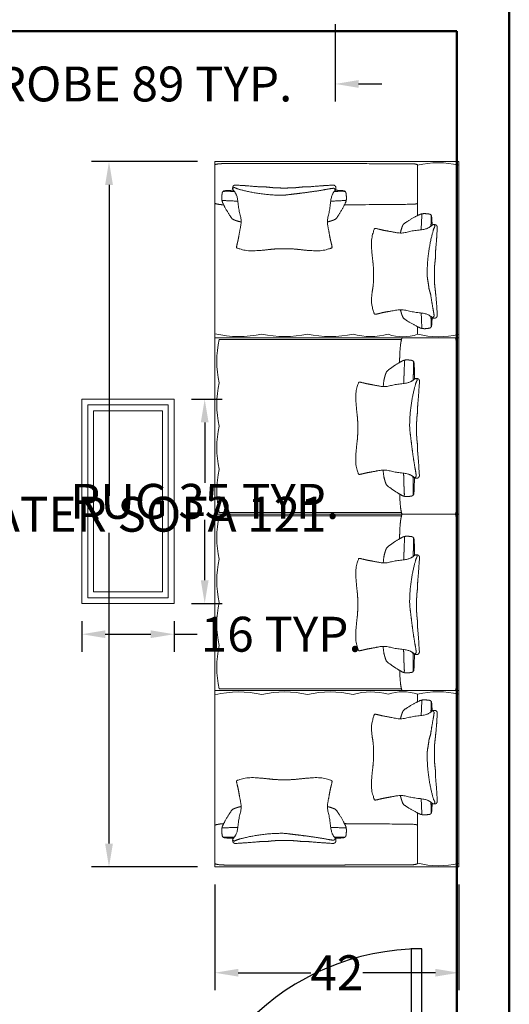
# Model space of a CAD drawing. Units: inches. Extents: x -466983 to 1020, y 324 to 318697.
# Tile 40 of 97: x 908 to 992, y 658 to 827. Entities that reach past the tile are written whole.
import ezdxf

# ---------------------------------------------------------------- set-up
doc = ezdxf.new("R2010")
doc.units = ezdxf.units.IN
doc.header["$MEASUREMENT"] = 0
for name, color, linetype, lineweight in [('A-ANNO-DIMS', 2, 'Continuous', 18), ('A-DOOR', 3, 'Continuous', 25), ('A-FURN', 8, 'Continuous', 18), ('A-WALL', 7, 'Continuous', 50)]:
    doc.layers.add(name, color=color, linetype=linetype, lineweight=lineweight)
doc.styles.get("Standard").update_dxf_attribs({"font": 'arial.ttf'})
doc.dimstyles.get("Standard").update_dxf_attribs({"dimtxt": 6, "dimasz": 4, "dimexe": 3, "dimexo": 3, "dimgap": 0.09, "dimtad": 0, "dimtih": 1, "dimtoh": 1, "dimdec": 1, "dimzin": 0, "dimdsep": 46, "dimlunit": 3, "dimtxsty": 'Standard', "dimcen": 0.09, "dimadec": 0, "dimazin": 0, "dimtfac": 1, "dimtdec": 1, "dimtofl": 0, "dimtmove": 0, "dimatfit": 3, "dimfxl": 1, "dimtolj": 1, "dimtzin": 0, "dimarcsym": 0})

# ---------------------------------------------------------------- blocks, each defined once
blk = doc.blocks.new('4 Seater Sofa Drawing')
for p, q in [((2474.13, 1022.64), (2521.12, 1022.64)), ((2474.13, 957.71), (2474.13, 1022.64)), ((2474.13, 1022.64), (2521.12, 1022.64)), ((2474.13, 957.71), (2474.13, 1022.64)), ((2568.11, 1022.64), (2521.12, 1022.64)), ((2521.12, 1022.64), (2521.12, 957.71)), ((2521.12, 1022.64), (2521.12, 957.71)), ((2521.12, 1022.64), (2521.12, 957.71)), ((2568.11, 957.71), (2568.11, 1022.64)), ((2615.09, 1022.64), (2568.11, 1022.64)), ((2568.11, 1022.64), (2568.11, 957.71)), ((2615.09, 957.71), (2615.09, 1022.64)), ((2662.08, 1022.64), (2615.09, 1022.64)), ((2615.09, 1022.64), (2615.09, 957.71)), ((2662.08, 957.71), (2662.08, 1022.64)), ((2485.15, 1011.7), (2488.51, 1011.7)), ((2518.14, 1011.7), (2520.13, 1011.7)), ((2618.07, 1011.7), (2616.08, 1011.7)), ((2651.06, 1011.7), (2647.71, 1011.7)), ((2521.57, 1007.39), (2521.57, 958.85)), ((2567.65, 1007.4), (2567.65, 986.81)), ((2568.56, 1007.39), (2568.56, 958.85)), ((2614.64, 1007.4), (2614.64, 986.81)), ((2567.65, 958.85), (2567.65, 986.81)), ((2614.64, 958.85), (2614.64, 986.81)), ((2521.12, 957.71), (2474.13, 957.71)), ((2521.12, 957.71), (2474.13, 957.71)), ((2521.12, 957.71), (2568.11, 957.71)), ((2568.11, 957.71), (2615.09, 957.71)), ((2615.09, 957.71), (2662.08, 957.71))]:
    blk.add_line(p, q)
at = {"extrusion": (0, 0, -1)}
for p, q in [((2568.11, 1022.64), (2521.12, 1022.64)), ((2521.12, 1022.64), (2521.12, 957.71)), ((2568.11, 957.71), (2568.11, 1022.64)), ((2615.09, 1022.64), (2568.11, 1022.64)), ((2568.11, 1022.64), (2568.11, 957.71)), ((2615.09, 957.71), (2615.09, 1022.64)), ((2662.08, 1022.64), (2615.09, 1022.64)), ((2615.09, 1022.64), (2615.09, 957.71)), ((2662.08, 957.71), (2662.08, 1022.64)), ((2521.12, 957.71), (2568.11, 957.71)), ((2568.11, 957.71), (2615.09, 957.71)), ((2615.09, 957.71), (2662.08, 957.71))]:
    blk.add_line(p, q, dxfattribs=at)
for centre, radius, start, end in [((2497.81, 1017.25), 23.36, 166.6748, 193.7611), ((2497.44, 1017.25), 23.36, 346.2389, 13.3252), ((2638.77, 1017.25), 23.36, 166.6748, 193.7611), ((2638.4, 1017.25), 23.36, 346.2389, 13.3252), ((2508.99, 1007.76), 11.82, 340.5487, 19.4513), ((2627.22, 1007.76), 11.82, 160.5487, 199.4513), ((2503.6, 999.25), 17.15, 343.8796, 15.4668), ((2632.61, 999.25), 17.15, 164.5332, 196.1204), ((2493.1, 988.42), 27.66, 347.3212, 12.6788), ((2643.12, 988.42), 27.66, 167.3212, 192.6788), ((2493.1, 976.28), 27.66, 347.3212, 12.6788), ((2643.12, 976.28), 27.66, 167.3212, 192.6788), ((2493.1, 964.14), 27.66, 346.5695, 12.6788), ((2643.12, 964.14), 27.66, 167.3212, 193.4305), ((2527.33, 984.45), 26.24, 257.3212, 282.6788), ((2538.86, 984.48), 26.27, 257.3272, 282.6647), ((2550.37, 984.48), 26.27, 257.3353, 282.6728), ((2561.9, 984.45), 26.24, 257.3212, 282.6788), ((2574.32, 984.45), 26.24, 257.3212, 282.6788), ((2585.84, 984.48), 26.27, 257.3272, 282.6647), ((2597.36, 984.48), 26.27, 257.3353, 282.6728), ((2608.88, 984.45), 26.24, 257.3212, 282.6788)]:
    blk.add_arc(centre, radius, start, end)
for points in [[(2522.19, 1022), (2521.12, 1021.86), (2521.12, 1021.69)], [(2521.12, 1021.69), (2521.12, 1012.51), (2521.12, 1007.6)], [(2530.42, 1022.1), (2524.11, 1022.1), (2523.25, 1022.08), (2522.69, 1022.05), (2522.19, 1022)], [(2539.72, 1022.1), (2535.07, 1022.1), (2530.42, 1022.1)], [(2558.8, 1022.1), (2549.26, 1022.1), (2539.72, 1022.1)], [(2567.04, 1022), (2566.54, 1022.05), (2565.98, 1022.08), (2565.12, 1022.1), (2558.8, 1022.1)], [(2568.11, 1021.69), (2568.11, 1021.86), (2567.04, 1022)], [(2569.17, 1022), (2568.11, 1021.86), (2568.11, 1021.69)], [(2568.11, 1007.6), (2568.11, 1012.51), (2568.11, 1021.69)], [(2568.11, 1021.69), (2568.11, 1012.51), (2568.11, 1007.6)], [(2577.41, 1022.1), (2571.1, 1022.1), (2570.23, 1022.08), (2569.67, 1022.05), (2569.17, 1022)], [(2586.7, 1022.1), (2582.06, 1022.1), (2577.41, 1022.1)], [(2605.79, 1022.1), (2596.25, 1022.1), (2586.7, 1022.1)], [(2614.03, 1022), (2613.53, 1022.05), (2612.97, 1022.08), (2612.1, 1022.1), (2605.79, 1022.1)], [(2615.09, 1021.69), (2615.09, 1021.86), (2614.03, 1022)], [(2615.09, 1007.6), (2615.09, 1012.51), (2615.09, 1021.69)], [(2501.5, 999.85), (2500.87, 999.78), (2498.56, 999.52), (2494.94, 999.32), (2492.12, 1000.1), (2491.9, 1000.31), (2492.12, 1001.33), (2492.44, 1002.59), (2492.75, 1004.42), (2493.33, 1007.39), (2492.57, 1010.18), (2492.19, 1013.75), (2491.52, 1015.06), (2490.91, 1015.73), (2490.9, 1016.23), (2491.01, 1016.65), (2491.47, 1016.97), (2491.84, 1016.93)], [(2491.37, 1016.31), (2491.29, 1016.29), (2490.91, 1016.08)], [(2491.84, 1016.93), (2493.92, 1016.78), (2494.29, 1016.78), (2497.41, 1016.52), (2498.38, 1016.42), (2499.92, 1016.45), (2500.85, 1016.32)], [(2500.85, 1016.32), (2501.67, 1016.22), (2502.67, 1016.17)], [(2505.99, 1016.17), (2506.99, 1016.22), (2507.81, 1016.32)], [(2514.92, 1016.93), (2515.29, 1016.97), (2515.75, 1016.65), (2515.86, 1016.23), (2515.85, 1015.73), (2515.24, 1015.06), (2514.57, 1013.75), (2514.2, 1010.18), (2513.43, 1007.39), (2514.01, 1004.42), (2514.32, 1002.59), (2514.64, 1001.33), (2514.87, 1000.31), (2514.64, 1000.1), (2511.82, 999.32), (2509.24, 999.52), (2507.79, 999.78), (2507.16, 999.85)], [(2507.81, 1016.32), (2508.73, 1016.45), (2509.42, 1016.42), (2509.36, 1016.52), (2512.47, 1016.78), (2512.84, 1016.78), (2514.92, 1016.93)], [(2515.74, 1015.66), (2515.41, 1016.03), (2515.29, 1016.08)], [(2621.29, 1016.93), (2620.92, 1016.97), (2620.46, 1016.65), (2620.36, 1016.23), (2620.37, 1015.73), (2620.97, 1015.06), (2621.64, 1013.75), (2622.02, 1010.18), (2622.78, 1007.39), (2622.2, 1004.42), (2621.89, 1002.59), (2621.58, 1001.33), (2621.35, 1000.31), (2621.57, 1000.1), (2624.39, 999.32), (2626.97, 999.52), (2628.43, 999.78), (2629.06, 999.85)], [(2620.47, 1015.66), (2620.81, 1016.03), (2620.93, 1016.08)], [(2628.41, 1016.32), (2627.48, 1016.45), (2626.79, 1016.42), (2626.86, 1016.52), (2623.74, 1016.78), (2623.37, 1016.78), (2621.29, 1016.93)], [(2630.23, 1016.17), (2629.23, 1016.22), (2628.41, 1016.32)], [(2635.37, 1016.32), (2634.55, 1016.22), (2633.55, 1016.17)], [(2634.72, 999.85), (2635.35, 999.78), (2637.65, 999.52), (2641.28, 999.32), (2644.09, 1000.1), (2644.32, 1000.31), (2644.09, 1001.33), (2643.78, 1002.59), (2643.47, 1004.42), (2642.89, 1007.39), (2643.65, 1010.18), (2644.03, 1013.75), (2644.69, 1015.06), (2645.3, 1015.73), (2645.31, 1016.23), (2645.21, 1016.65), (2644.74, 1016.97), (2644.38, 1016.93)], [(2644.38, 1016.93), (2642.3, 1016.78), (2641.93, 1016.78), (2638.81, 1016.52), (2637.83, 1016.42), (2636.29, 1016.45), (2635.37, 1016.32)], [(2644.85, 1016.31), (2644.93, 1016.29), (2645.31, 1016.08)], [(2505.36, 1014.32), (2505.01, 1014.28), (2504.66, 1014.25)], [(2507.98, 1014.72), (2506.44, 1014.53), (2505.36, 1014.32)], [(2509.58, 1015.18), (2508.66, 1014.9), (2507.98, 1014.72)], [(2626.63, 1015.18), (2627.56, 1014.9), (2628.24, 1014.72)], [(2628.24, 1014.72), (2629.77, 1014.53), (2630.86, 1014.32)], [(2630.86, 1014.32), (2631.21, 1014.28), (2631.56, 1014.25)], [(2474.62, 984.72), (2474.62, 991.35), (2474.64, 992.25), (2474.67, 992.84), (2474.72, 1010.58)], [(2474.72, 1010.58), (2474.87, 1011.7), (2475.04, 1011.7)], [(2475.04, 1011.7), (2480.12, 1011.7), (2485.19, 1011.7)], [(2485.19, 1011.7), (2485.33, 1011.7), (2485.46, 1010.93)], [(2485.46, 1010.93), (2485.55, 1010.63), (2485.64, 992.78)], [(2488.12, 1012.61), (2488.12, 1012.58), (2488.13, 1012.54)], [(2518.53, 1012.61), (2518.53, 1012.58), (2518.52, 1012.54)], [(2542.13, 995.65), (2541.53, 995.58), (2539.29, 995.34), (2535.79, 995.15), (2533.06, 995.91), (2532.85, 996.11), (2533.07, 997.1), (2533.37, 998.32), (2533.68, 1000.08), (2534.24, 1002.96), (2533.51, 1005.66), (2533.15, 1009.12), (2532.51, 1010.38), (2531.92, 1011.04), (2531.91, 1011.51), (2532.01, 1011.92), (2532.46, 1012.23), (2532.81, 1012.19)], [(2532.36, 1011.59), (2532.28, 1011.57), (2531.91, 1011.37)], [(2532.81, 1012.19), (2534.83, 1012.04), (2535.19, 1012.04), (2538.2, 1011.79), (2539.14, 1011.69), (2540.64, 1011.71), (2541.53, 1011.58)], [(2541.53, 1011.58), (2542.32, 1011.49), (2543.29, 1011.44)], [(2547.14, 1011.43), (2548.11, 1011.48), (2548.9, 1011.57)], [(2557.62, 1012.16), (2557.98, 1012.19), (2558.43, 1011.88), (2558.53, 1011.47), (2558.51, 1010.99), (2557.92, 1010.34), (2557.28, 1009.08), (2556.91, 1005.62), (2556.17, 1002.92), (2556.72, 1000.05), (2557.02, 998.28), (2557.32, 997.06), (2557.54, 996.07), (2557.32, 995.87), (2554.6, 995.12), (2551.09, 995.32), (2548.86, 995.57), (2548.25, 995.64)], [(2548.9, 1011.57), (2549.8, 1011.7), (2551.29, 1011.67), (2552.23, 1011.77), (2555.25, 1012.01), (2555.61, 1012.01), (2557.62, 1012.16)], [(2558.41, 1010.92), (2558.09, 1011.29), (2557.97, 1011.33)], [(2589.12, 995.65), (2588.51, 995.58), (2586.28, 995.34), (2582.77, 995.15), (2580.05, 995.91), (2579.83, 996.11), (2580.06, 997.1), (2580.36, 998.32), (2580.66, 1000.08), (2581.23, 1002.96), (2580.5, 1005.66), (2580.14, 1009.12), (2579.49, 1010.38), (2578.9, 1011.04), (2578.9, 1011.51), (2579, 1011.92), (2579.45, 1012.23), (2579.8, 1012.19)], [(2579.34, 1011.59), (2579.27, 1011.57), (2578.9, 1011.37)], [(2579.8, 1012.19), (2581.81, 1012.04), (2582.17, 1012.04), (2585.19, 1011.79), (2586.13, 1011.69), (2587.63, 1011.71), (2588.52, 1011.58)], [(2588.52, 1011.58), (2589.31, 1011.49), (2590.28, 1011.44)], [(2594.13, 1011.43), (2595.1, 1011.48), (2595.89, 1011.57)], [(2604.61, 1012.16), (2604.96, 1012.19), (2605.41, 1011.88), (2605.51, 1011.47), (2605.5, 1010.99), (2604.91, 1010.34), (2604.26, 1009.08), (2603.89, 1005.62), (2603.15, 1002.92), (2603.71, 1000.05), (2604.01, 998.28), (2604.31, 997.06), (2604.53, 996.07), (2604.31, 995.87), (2601.58, 995.12), (2598.08, 995.32), (2595.85, 995.57), (2595.24, 995.64)], [(2595.89, 1011.57), (2596.78, 1011.7), (2598.28, 1011.67), (2599.22, 1011.77), (2602.24, 1012.01), (2602.6, 1012.01), (2604.61, 1012.16)], [(2605.4, 1010.92), (2605.08, 1011.29), (2604.96, 1011.33)], [(2617.68, 1012.61), (2617.68, 1012.58), (2617.69, 1012.54)], [(2648.1, 1012.61), (2648.1, 1012.58), (2648.09, 1012.54)], [(2650.76, 1010.93), (2650.66, 1010.63), (2650.58, 992.78)], [(2651.03, 1011.7), (2650.88, 1011.7), (2650.76, 1010.93)], [(2661.17, 1011.7), (2656.1, 1011.7), (2651.03, 1011.7)], [(2661.49, 1010.58), (2661.34, 1011.7), (2661.17, 1011.7)], [(2661.6, 984.72), (2661.59, 991.35), (2661.58, 992.25), (2661.55, 992.84), (2661.49, 1010.58)], [(2521.12, 1007.6), (2521.12, 1007.47), (2521.84, 1007.34)], [(2527.1, 1008.02), (2527.1, 1007.99), (2527.11, 1007.95)], [(2563.27, 1007.96), (2563.27, 1007.94), (2563.26, 1007.89)], [(2567.38, 1007.34), (2568.11, 1007.47), (2568.11, 1007.6)], [(2568.11, 1007.6), (2568.11, 1007.47), (2568.83, 1007.34)], [(2574.09, 1008.02), (2574.09, 1007.99), (2574.1, 1007.95)], [(2610.26, 1007.96), (2610.26, 1007.94), (2610.25, 1007.89)], [(2614.37, 1007.34), (2615.09, 1007.47), (2615.09, 1007.6)], [(2484.71, 992.62), (2484.74, 992.62), (2484.78, 992.61)], [(2485.64, 992.78), (2485.67, 992.51), (2485.71, 992.19)], [(2650.58, 992.78), (2650.54, 992.51), (2650.51, 992.19)], [(2651.5, 992.62), (2651.48, 992.62), (2651.43, 992.61)], [(2480.39, 989.01), (2480.35, 989.38), (2480.67, 989.84), (2481.09, 989.95), (2481.59, 989.94), (2482.26, 989.33), (2483.57, 988.66), (2487.14, 988.29), (2489.93, 987.52), (2492.9, 988.1), (2494.73, 988.41), (2495.99, 988.73), (2497.01, 988.96), (2497.22, 988.73), (2498, 985.91), (2497.8, 982.29), (2497.54, 979.98), (2497.47, 979.35)], [(2481.66, 989.83), (2481.29, 989.5), (2481.24, 989.38)], [(2655.83, 989.01), (2655.87, 989.38), (2655.54, 989.84), (2655.12, 989.95), (2654.63, 989.94), (2653.95, 989.33), (2652.65, 988.66), (2649.07, 988.29), (2646.28, 987.52), (2643.31, 988.1), (2641.49, 988.41), (2640.23, 988.73), (2639.2, 988.96), (2639, 988.73), (2638.21, 985.91), (2638.41, 982.29), (2638.67, 979.98), (2638.74, 979.35)], [(2654.55, 989.83), (2654.93, 989.5), (2654.97, 989.38)], [(2481, 980), (2480.87, 980.93), (2480.9, 982.47), (2480.8, 983.45), (2480.54, 986.56), (2480.54, 986.93), (2480.39, 989.01)], [(2655.21, 980), (2655.34, 980.93), (2655.32, 982.47), (2655.42, 983.45), (2655.67, 986.56), (2655.68, 986.93), (2655.83, 989.01)], [(2474.62, 976.28), (2474.62, 980.5), (2474.62, 984.72)], [(2661.6, 976.28), (2661.6, 980.5), (2661.6, 984.72)], [(2481.15, 978.18), (2481.1, 979.18), (2481, 980)], [(2655.06, 978.18), (2655.12, 979.18), (2655.21, 980)], [(2474.62, 967.83), (2474.62, 972.05), (2474.62, 976.28)], [(2661.6, 967.83), (2661.6, 972.05), (2661.6, 976.28)], [(2481, 972.38), (2481.1, 973.2), (2481.15, 974.2)], [(2655.21, 972.38), (2655.12, 973.2), (2655.06, 974.2)], [(2497.47, 973.03), (2497.54, 972.4), (2497.8, 970.1), (2498, 966.47), (2497.22, 963.66), (2497.01, 963.43), (2495.99, 963.66), (2494.73, 963.97), (2492.9, 964.28), (2489.93, 964.86), (2487.14, 964.1), (2483.57, 963.73), (2482.26, 963.06), (2481.59, 962.45), (2481.09, 962.44), (2480.67, 962.54), (2480.35, 963.01), (2480.39, 963.37)], [(2480.39, 963.37), (2480.54, 965.45), (2480.54, 965.82), (2480.8, 968.94), (2480.9, 969.92), (2480.87, 971.46), (2481, 972.38)], [(2638.74, 973.03), (2638.67, 972.4), (2638.41, 970.1), (2638.21, 966.47), (2639, 963.66), (2639.2, 963.43), (2640.23, 963.66), (2641.49, 963.97), (2643.31, 964.28), (2646.28, 964.86), (2649.07, 964.1), (2652.65, 963.73), (2653.95, 963.06), (2654.63, 962.45), (2655.12, 962.44), (2655.54, 962.54), (2655.87, 963.01), (2655.83, 963.37)], [(2655.83, 963.37), (2655.68, 965.45), (2655.67, 965.82), (2655.42, 968.94), (2655.32, 969.92), (2655.34, 971.46), (2655.21, 972.38)], [(2474.72, 958.83), (2474.67, 959.71), (2474.64, 960.3), (2474.62, 961.2), (2474.62, 967.83)], [(2661.49, 958.83), (2661.55, 959.71), (2661.58, 960.3), (2661.59, 961.2), (2661.6, 967.83)], [(2481.01, 962.9), (2481.03, 962.82), (2481.24, 962.44)], [(2655.21, 962.9), (2655.18, 962.82), (2654.97, 962.44)], [(2475.04, 957.71), (2474.87, 957.71), (2474.72, 958.83)], [(2485.19, 957.71), (2480.12, 957.71), (2475.04, 957.71)], [(2484.71, 959.66), (2484.74, 959.65), (2484.78, 959.67)], [(2485.46, 958.47), (2485.33, 957.71), (2485.19, 957.71)], [(2485.64, 959.77), (2485.55, 958.78), (2485.46, 958.47)], [(2485.67, 960.07), (2485.66, 959.91), (2485.64, 959.77)], [(2650.54, 960.07), (2650.56, 959.91), (2650.58, 959.77)], [(2650.58, 959.77), (2650.66, 958.78), (2650.76, 958.47)], [(2650.76, 958.47), (2650.88, 957.71), (2651.03, 957.71)], [(2651.03, 957.71), (2656.1, 957.71), (2661.17, 957.71)], [(2651.5, 959.66), (2651.48, 959.65), (2651.43, 959.67)], [(2661.17, 957.71), (2661.34, 957.71), (2661.49, 958.83)]]:
    blk.add_open_spline(points, degree=2)
for points, knots in [([(2488.13, 1012.54), (2487.94, 1013.32), (2488.07, 1014.32), (2488.12, 1014.95), (2488.42, 1015.35), (2488.86, 1015.43), (2489.39, 1015.48), (2489.76, 1015.51), (2491.09, 1015.55)], [6, 6, 6, 7, 8, 9, 10, 11, 11, 12, 12, 12]), ([(2504.66, 1014.25), (2502.17, 1014.18), (2499.43, 1014.49), (2496.7, 1014.81), (2494.57, 1015.31), (2492.43, 1015.82), (2492, 1016.01), (2491.58, 1016.2), (2491.44, 1016.28), (2491.4, 1016.31), (2491.37, 1016.31)], [6, 6, 6, 7, 7, 8, 8, 9, 9, 10, 10, 11, 11, 11]), ([(2502.67, 1016.17), (2503.43, 1016.15), (2504.2, 1016.15), (2504.66, 1016.15), (2505.11, 1016.15), (2505.89, 1016.15), (2505.99, 1016.17)], [24, 24, 24, 25, 25, 27, 27, 28, 28, 28]), ([(2515.29, 1016.08), (2514.99, 1016.09), (2513.38, 1015.79), (2511.55, 1015.46), (2509.58, 1015.18)], [1, 1, 1, 2, 2, 3, 3, 3]), ([(2515.67, 1015.55), (2516.91, 1015.51), (2517.26, 1015.48), (2517.79, 1015.43), (2518.23, 1015.35), (2518.53, 1014.95), (2518.58, 1014.32), (2518.71, 1013.32), (2518.52, 1012.54)], [0, 0, 0, 1, 1, 2, 3, 4, 5, 6, 6, 6]), ([(2620.55, 1015.55), (2619.31, 1015.51), (2618.95, 1015.48), (2618.43, 1015.43), (2617.98, 1015.35), (2617.68, 1014.95), (2617.63, 1014.32), (2617.51, 1013.32), (2617.69, 1012.54)], [0, 0, 0, 1, 1, 2, 3, 4, 5, 6, 6, 6]), ([(2620.93, 1016.08), (2621.22, 1016.09), (2622.84, 1015.79), (2624.67, 1015.46), (2626.63, 1015.18)], [1, 1, 1, 2, 2, 3, 3, 3]), ([(2633.55, 1016.17), (2632.79, 1016.15), (2632.01, 1016.15), (2631.56, 1016.15), (2631.1, 1016.15), (2630.33, 1016.15), (2630.23, 1016.17)], [24, 24, 24, 25, 25, 27, 27, 28, 28, 28]), ([(2631.56, 1014.25), (2634.05, 1014.18), (2636.78, 1014.49), (2639.51, 1014.81), (2641.64, 1015.31), (2643.79, 1015.82), (2644.22, 1016.01), (2644.64, 1016.2), (2644.78, 1016.28), (2644.82, 1016.31), (2644.85, 1016.31)], [6, 6, 6, 7, 7, 8, 8, 9, 9, 10, 10, 11, 11, 11]), ([(2648.09, 1012.54), (2648.27, 1013.32), (2648.15, 1014.32), (2648.1, 1014.95), (2647.8, 1015.35), (2647.36, 1015.43), (2646.83, 1015.48), (2646.46, 1015.51), (2645.12, 1015.55)], [6, 6, 6, 7, 8, 9, 10, 11, 11, 12, 12, 12]), ([(2492.29, 1012.65), (2492.22, 1012.65), (2492.16, 1012.66), (2491.4, 1012.67), (2489.25, 1012.77), (2488.49, 1012.82), (2488.14, 1012.77), (2488.12, 1012.61)], [0, 0, 0, 1, 1, 2, 3, 4, 5, 5, 5]), ([(2488.37, 1015.26), (2489.22, 1015.27), (2489.74, 1015.27), (2490.32, 1015.27), (2491.35, 1015.24)], [0, 0, 0, 1, 1, 2, 2, 2]), ([(2518.53, 1012.61), (2518.51, 1012.77), (2518.16, 1012.82), (2517.4, 1012.77), (2515.25, 1012.67), (2514.49, 1012.66), (2514.48, 1012.66), (2514.47, 1012.66)], [0, 0, 0, 1, 2, 3, 4, 4, 5, 5, 5]), ([(2515.42, 1015.24), (2516.36, 1015.27), (2516.91, 1015.27), (2517.43, 1015.27), (2518.28, 1015.26)], [0, 0, 0, 1, 1, 2, 2, 2]), ([(2617.68, 1012.61), (2617.7, 1012.77), (2618.06, 1012.82), (2618.81, 1012.77), (2620.96, 1012.67), (2621.72, 1012.66), (2621.73, 1012.66), (2621.75, 1012.66)], [0, 0, 0, 1, 2, 3, 4, 4, 5, 5, 5]), ([(2620.8, 1015.24), (2619.86, 1015.27), (2619.31, 1015.27), (2618.78, 1015.27), (2617.93, 1015.26)], [0, 0, 0, 1, 1, 2, 2, 2]), ([(2643.92, 1012.65), (2643.99, 1012.65), (2644.06, 1012.66), (2644.82, 1012.67), (2646.97, 1012.77), (2647.73, 1012.82), (2648.08, 1012.77), (2648.1, 1012.61)], [0, 0, 0, 1, 1, 2, 3, 4, 5, 5, 5]), ([(2647.85, 1015.26), (2647, 1015.27), (2646.47, 1015.27), (2645.89, 1015.27), (2644.87, 1015.24)], [0, 0, 0, 1, 1, 2, 2, 2]), ([(2493.16, 1007.11), (2492.76, 1007.18), (2492.56, 1007.24), (2491.72, 1007.49), (2491.17, 1007.71), (2490.75, 1007.93), (2489.53, 1009.76), (2488.82, 1011.1), (2488.2, 1012.26), (2488.13, 1012.54)], [0, 0, 0, 1, 1, 2, 3, 4, 5, 5, 6, 6, 6]), ([(2518.52, 1012.54), (2518.45, 1012.26), (2517.83, 1011.1), (2517.12, 1009.76), (2515.9, 1007.93), (2515.48, 1007.71), (2514.93, 1007.49), (2514.09, 1007.24), (2513.92, 1007.18), (2513.6, 1007.13)], [6, 6, 6, 7, 7, 8, 9, 10, 11, 11, 12, 12, 12]), ([(2527.11, 1007.95), (2526.91, 1008.71), (2527.05, 1009.67), (2527.11, 1010.29), (2527.43, 1010.67), (2527.92, 1010.75), (2529.08, 1010.84), (2531.81, 1010.89), (2531.94, 1010.89), (2532.07, 1010.89)], [6, 6, 6, 7, 8, 9, 10, 11, 12, 12, 13, 13, 13]), ([(2527.38, 1010.58), (2528.31, 1010.59), (2528.89, 1010.59), (2529.6, 1010.59), (2530.92, 1010.55), (2531.62, 1010.53), (2532.39, 1010.48)], [0, 0, 0, 1, 1, 2, 2, 3, 3, 3]), ([(2545.21, 1009.58), (2542.81, 1009.52), (2540.16, 1009.82), (2537.52, 1010.13), (2535.46, 1010.62), (2533.39, 1011.12), (2532.97, 1011.3), (2532.56, 1011.49), (2532.43, 1011.57), (2532.39, 1011.59), (2532.36, 1011.59)], [6, 6, 6, 7, 7, 8, 8, 9, 9, 10, 10, 11, 11, 11]), ([(2543.29, 1011.44), (2544.03, 1011.42), (2544.78, 1011.42), (2545.22, 1011.42), (2545.66, 1011.42), (2546.41, 1011.42), (2547.14, 1011.43)], [24, 24, 24, 25, 25, 27, 27, 28, 28, 28]), ([(2557.97, 1011.33), (2557.69, 1011.34), (2556.13, 1011.06), (2554.35, 1010.73), (2552.45, 1010.47), (2550.55, 1010.2), (2549.06, 1010.03), (2547.58, 1009.85), (2545.89, 1009.65), (2545.55, 1009.6), (2545.21, 1009.58)], [1, 1, 1, 2, 2, 3, 3, 4, 4, 5, 5, 6, 6, 6]), ([(2558.04, 1010.45), (2558.78, 1010.49), (2559.46, 1010.51), (2560.78, 1010.54), (2561.49, 1010.54), (2562.07, 1010.54), (2563, 1010.53)], [0, 0, 0, 1, 1, 2, 2, 3, 3, 3]), ([(2558.37, 1010.85), (2558.47, 1010.85), (2558.57, 1010.84), (2561.3, 1010.79), (2562.46, 1010.69), (2562.94, 1010.62), (2563.27, 1010.23), (2563.33, 1009.62), (2563.46, 1008.65), (2563.26, 1007.89)], [0, 0, 0, 1, 1, 2, 3, 4, 5, 6, 7, 7, 7]), ([(2574.1, 1007.95), (2573.9, 1008.71), (2574.03, 1009.67), (2574.09, 1010.29), (2574.42, 1010.67), (2574.91, 1010.75), (2576.07, 1010.84), (2578.79, 1010.89), (2578.92, 1010.89), (2579.05, 1010.89)], [6, 6, 6, 7, 8, 9, 10, 11, 12, 12, 13, 13, 13]), ([(2574.37, 1010.58), (2575.3, 1010.59), (2575.87, 1010.59), (2576.59, 1010.59), (2577.9, 1010.55), (2578.61, 1010.53), (2579.38, 1010.48)], [0, 0, 0, 1, 1, 2, 2, 3, 3, 3]), ([(2592.2, 1009.58), (2589.79, 1009.52), (2587.15, 1009.82), (2584.51, 1010.13), (2582.44, 1010.62), (2580.37, 1011.12), (2579.95, 1011.3), (2579.55, 1011.49), (2579.41, 1011.57), (2579.37, 1011.59), (2579.34, 1011.59)], [6, 6, 6, 7, 7, 8, 8, 9, 9, 10, 10, 11, 11, 11]), ([(2590.28, 1011.44), (2591.01, 1011.42), (2591.76, 1011.42), (2592.2, 1011.42), (2592.64, 1011.42), (2593.4, 1011.42), (2594.13, 1011.43)], [24, 24, 24, 25, 25, 27, 27, 28, 28, 28]), ([(2604.96, 1011.33), (2604.68, 1011.34), (2603.11, 1011.06), (2601.34, 1010.73), (2599.44, 1010.47), (2597.54, 1010.2), (2596.05, 1010.03), (2594.57, 1009.85), (2592.88, 1009.65), (2592.54, 1009.6), (2592.2, 1009.58)], [1, 1, 1, 2, 2, 3, 3, 4, 4, 5, 5, 6, 6, 6]), ([(2605.03, 1010.45), (2605.77, 1010.49), (2606.45, 1010.51), (2607.77, 1010.54), (2608.48, 1010.54), (2609.05, 1010.54), (2609.99, 1010.53)], [0, 0, 0, 1, 1, 2, 2, 3, 3, 3]), ([(2605.35, 1010.85), (2605.46, 1010.85), (2605.56, 1010.84), (2608.29, 1010.79), (2609.45, 1010.69), (2609.93, 1010.62), (2610.26, 1010.23), (2610.32, 1009.62), (2610.45, 1008.65), (2610.25, 1007.89)], [0, 0, 0, 1, 1, 2, 3, 4, 5, 6, 7, 7, 7]), ([(2617.69, 1012.54), (2617.77, 1012.26), (2618.38, 1011.1), (2619.1, 1009.76), (2620.31, 1007.93), (2620.73, 1007.71), (2621.28, 1007.49), (2622.13, 1007.24), (2622.3, 1007.18), (2622.62, 1007.13)], [6, 6, 6, 7, 7, 8, 9, 10, 11, 11, 12, 12, 12]), ([(2643.05, 1007.11), (2643.46, 1007.18), (2643.65, 1007.24), (2644.5, 1007.49), (2645.05, 1007.71), (2645.47, 1007.93), (2646.69, 1009.76), (2647.4, 1011.1), (2648.01, 1012.26), (2648.09, 1012.54)], [0, 0, 0, 1, 1, 2, 3, 4, 5, 5, 6, 6, 6]), ([(2533.26, 1007.97), (2532.26, 1008.05), (2531.53, 1008.06), (2530.7, 1008.07), (2528.34, 1008.17), (2527.51, 1008.23), (2527.12, 1008.17), (2527.1, 1008.02)], [0, 0, 0, 1, 1, 2, 3, 4, 5, 5, 5]), ([(2534.08, 1002.53), (2532.46, 1002.68), (2531.97, 1002.81), (2531.04, 1003.06), (2530.44, 1003.28), (2529.98, 1003.49), (2528.64, 1005.26), (2527.86, 1006.56), (2527.19, 1007.68), (2527.11, 1007.95)], [0, 0, 0, 1, 1, 2, 3, 4, 5, 5, 6, 6, 6]), ([(2563.26, 1007.89), (2563.18, 1007.62), (2562.5, 1006.51), (2561.72, 1005.21), (2560.38, 1003.44), (2559.92, 1003.23), (2559.32, 1003.02), (2558.39, 1002.77), (2557.91, 1002.64), (2556.33, 1002.5)], [7, 7, 7, 8, 8, 9, 10, 11, 12, 12, 13, 13, 13]), ([(2563.27, 1007.96), (2563.25, 1008.11), (2562.86, 1008.17), (2562.03, 1008.12), (2559.67, 1008.02), (2558.84, 1008.02), (2558.13, 1008.01), (2557.16, 1007.94)], [0, 0, 0, 1, 2, 3, 4, 4, 5, 5, 5]), ([(2580.25, 1007.97), (2579.25, 1008.05), (2578.52, 1008.06), (2577.69, 1008.07), (2575.33, 1008.17), (2574.5, 1008.23), (2574.11, 1008.17), (2574.09, 1008.02)], [0, 0, 0, 1, 1, 2, 3, 4, 5, 5, 5]), ([(2581.07, 1002.53), (2579.44, 1002.68), (2578.95, 1002.81), (2578.03, 1003.06), (2577.43, 1003.28), (2576.96, 1003.49), (2575.63, 1005.26), (2574.85, 1006.56), (2574.18, 1007.68), (2574.1, 1007.95)], [0, 0, 0, 1, 1, 2, 3, 4, 5, 5, 6, 6, 6]), ([(2610.25, 1007.89), (2610.16, 1007.62), (2609.49, 1006.51), (2608.7, 1005.21), (2607.37, 1003.44), (2606.9, 1003.23), (2606.3, 1003.02), (2605.37, 1002.77), (2604.89, 1002.64), (2603.32, 1002.5)], [7, 7, 7, 8, 8, 9, 10, 11, 12, 12, 13, 13, 13]), ([(2610.26, 1007.96), (2610.24, 1008.11), (2609.85, 1008.17), (2609.02, 1008.12), (2606.66, 1008.02), (2605.83, 1008.02), (2605.12, 1008.01), (2604.15, 1007.94)], [0, 0, 0, 1, 2, 3, 4, 4, 5, 5, 5]), ([(2521.84, 1007.34), (2522.14, 1007.25), (2522.74, 1007.17), (2523.83, 1007.02), (2525.69, 1006.94), (2526.64, 1006.9), (2527.68, 1006.88)], [17, 17, 17, 18, 18, 19, 19, 20, 20, 20]), ([(2562.74, 1006.91), (2563.14, 1006.92), (2563.54, 1006.94), (2565.4, 1007.02), (2566.48, 1007.17), (2567.09, 1007.25), (2567.38, 1007.34)], [0, 0, 0, 1, 1, 2, 2, 3, 3, 3]), ([(2568.83, 1007.34), (2569.12, 1007.25), (2569.73, 1007.17), (2570.81, 1007.02), (2572.68, 1006.94), (2573.63, 1006.9), (2574.66, 1006.88)], [17, 17, 17, 18, 18, 19, 19, 20, 20, 20]), ([(2609.73, 1006.91), (2610.13, 1006.92), (2610.52, 1006.94), (2612.39, 1007.02), (2613.47, 1007.17), (2614.08, 1007.25), (2614.37, 1007.34)], [0, 0, 0, 1, 1, 2, 2, 3, 3, 3]), ([(2504.66, 999.97), (2504.42, 999.97), (2504.19, 999.97), (2502.8, 999.97), (2501.5, 999.85)], [0, 0, 0, 1, 1, 2, 2, 2]), ([(2507.16, 999.85), (2505.85, 999.97), (2505.12, 999.97), (2504.89, 999.97), (2504.66, 999.97)], [50, 50, 50, 51, 51, 52, 52, 52]), ([(2629.06, 999.85), (2630.36, 999.97), (2631.09, 999.97), (2631.32, 999.97), (2631.56, 999.97)], [50, 50, 50, 51, 51, 52, 52, 52]), ([(2631.56, 999.97), (2631.79, 999.97), (2632.02, 999.97), (2633.41, 999.97), (2634.72, 999.85)], [0, 0, 0, 1, 1, 2, 2, 2]), ([(2545.19, 995.76), (2544.97, 995.76), (2544.74, 995.76), (2543.4, 995.77), (2542.13, 995.65)], [0, 0, 0, 1, 1, 2, 2, 2]), ([(2548.25, 995.64), (2546.99, 995.76), (2545.64, 995.76), (2545.42, 995.76), (2545.19, 995.76)], [50, 50, 50, 51, 51, 52, 52, 52]), ([(2592.18, 995.76), (2591.95, 995.76), (2591.73, 995.76), (2590.39, 995.77), (2589.12, 995.65)], [0, 0, 0, 1, 1, 2, 2, 2]), ([(2595.24, 995.64), (2593.97, 995.76), (2592.63, 995.76), (2592.4, 995.76), (2592.18, 995.76)], [50, 50, 50, 51, 51, 52, 52, 52]), ([(2481.77, 989.76), (2481.81, 991), (2481.84, 991.35), (2481.89, 991.88), (2481.97, 992.32), (2482.37, 992.62), (2483, 992.67), (2484, 992.8), (2484.78, 992.61)], [0, 0, 0, 1, 1, 2, 3, 4, 5, 6, 6, 6]), ([(2482.08, 989.51), (2482.05, 990.45), (2482.05, 991), (2482.05, 991.52), (2482.06, 992.37)], [0, 0, 0, 1, 1, 2, 2, 2]), ([(2484.71, 992.62), (2484.55, 992.6), (2484.5, 992.25), (2484.55, 991.49), (2484.65, 989.34), (2484.66, 988.58), (2484.66, 988.57), (2484.66, 988.56)], [0, 0, 0, 1, 2, 3, 4, 4, 5, 5, 5]), ([(2484.78, 992.61), (2485.06, 992.54), (2486.22, 991.92), (2487.56, 991.21), (2489.39, 989.99), (2489.61, 989.57), (2489.83, 989.02), (2490.08, 988.18), (2490.14, 988.01), (2490.19, 987.69)], [6, 6, 6, 7, 7, 8, 9, 10, 11, 11, 12, 12, 12]), ([(2651.43, 992.61), (2651.15, 992.54), (2650, 991.92), (2648.66, 991.21), (2646.83, 989.99), (2646.61, 989.57), (2646.39, 989.02), (2646.13, 988.18), (2646.08, 988.01), (2646.03, 987.69)], [6, 6, 6, 7, 7, 8, 9, 10, 11, 11, 12, 12, 12]), ([(2654.44, 989.76), (2654.41, 991), (2654.37, 991.35), (2654.32, 991.88), (2654.25, 992.32), (2653.85, 992.62), (2653.21, 992.67), (2652.22, 992.8), (2651.43, 992.61)], [0, 0, 0, 1, 1, 2, 3, 4, 5, 6, 6, 6]), ([(2651.5, 992.62), (2651.66, 992.6), (2651.72, 992.25), (2651.66, 991.49), (2651.56, 989.34), (2651.55, 988.58), (2651.55, 988.57), (2651.55, 988.56)], [0, 0, 0, 1, 2, 3, 4, 4, 5, 5, 5]), ([(2654.14, 989.51), (2654.17, 990.45), (2654.17, 991), (2654.17, 991.52), (2654.15, 992.37)], [0, 0, 0, 1, 1, 2, 2, 2]), ([(2481.24, 989.38), (2481.23, 989.08), (2481.53, 987.47), (2481.86, 985.64), (2482.14, 983.67), (2482.42, 981.71), (2482.6, 980.17), (2482.79, 978.64), (2483, 976.89), (2483.04, 976.54), (2483.07, 976.19)], [1, 1, 1, 2, 2, 3, 3, 4, 4, 5, 5, 6, 6, 6]), ([(2654.97, 989.38), (2654.99, 989.08), (2654.69, 987.47), (2654.35, 985.64), (2654.07, 983.67), (2653.8, 981.71), (2653.61, 980.17), (2653.43, 978.64), (2653.21, 976.89), (2653.17, 976.54), (2653.14, 976.19)], [1, 1, 1, 2, 2, 3, 3, 4, 4, 5, 5, 6, 6, 6]), ([(2497.47, 979.35), (2497.35, 978.05), (2497.35, 976.66), (2497.35, 976.43), (2497.35, 976.19)], [50, 50, 50, 51, 51, 52, 52, 52]), ([(2638.74, 979.35), (2638.86, 978.05), (2638.86, 976.66), (2638.86, 976.43), (2638.86, 976.19)], [50, 50, 50, 51, 51, 52, 52, 52]), ([(2483.07, 976.19), (2483.14, 973.7), (2482.83, 970.97), (2482.51, 968.24), (2482.01, 966.11), (2481.5, 963.97), (2481.31, 963.53), (2481.12, 963.11), (2481.04, 962.97), (2481.01, 962.93), (2481.01, 962.9)], [6, 6, 6, 7, 7, 8, 8, 9, 9, 10, 10, 11, 11, 11]), ([(2481.15, 974.2), (2481.17, 974.96), (2481.17, 975.74), (2481.17, 976.19), (2481.17, 976.65), (2481.17, 977.42), (2481.15, 978.18)], [24, 24, 24, 25, 25, 27, 27, 28, 28, 28]), ([(2497.35, 976.19), (2497.35, 975.96), (2497.35, 975.73), (2497.35, 974.34), (2497.47, 973.03)], [0, 0, 0, 1, 1, 2, 2, 2]), ([(2638.86, 976.19), (2638.86, 975.96), (2638.86, 975.73), (2638.86, 974.34), (2638.74, 973.03)], [0, 0, 0, 1, 1, 2, 2, 2]), ([(2653.14, 976.19), (2653.08, 973.7), (2653.39, 970.97), (2653.7, 968.24), (2654.21, 966.11), (2654.72, 963.97), (2654.91, 963.53), (2655.1, 963.11), (2655.18, 962.97), (2655.2, 962.93), (2655.21, 962.9)], [6, 6, 6, 7, 7, 8, 8, 9, 9, 10, 10, 11, 11, 11]), ([(2655.06, 974.2), (2655.05, 974.96), (2655.05, 975.74), (2655.05, 976.19), (2655.05, 976.65), (2655.05, 977.42), (2655.06, 978.18)], [24, 24, 24, 25, 25, 27, 27, 28, 28, 28]), ([(2484.67, 963.83), (2484.67, 963.76), (2484.66, 963.69), (2484.65, 962.93), (2484.55, 960.78), (2484.5, 960.03), (2484.55, 959.67), (2484.71, 959.66)], [0, 0, 0, 1, 1, 2, 3, 4, 5, 5, 5]), ([(2490.21, 964.7), (2490.14, 964.3), (2490.08, 964.1), (2489.83, 963.25), (2489.61, 962.71), (2489.39, 962.28), (2487.56, 961.07), (2486.22, 960.35), (2485.06, 959.74), (2484.78, 959.67)], [0, 0, 0, 1, 1, 2, 3, 4, 5, 5, 6, 6, 6]), ([(2646.01, 964.7), (2646.07, 964.3), (2646.13, 964.1), (2646.39, 963.25), (2646.61, 962.71), (2646.83, 962.28), (2648.66, 961.07), (2650, 960.35), (2651.15, 959.74), (2651.43, 959.67)], [0, 0, 0, 1, 1, 2, 3, 4, 5, 5, 6, 6, 6]), ([(2651.55, 963.83), (2651.55, 963.76), (2651.55, 963.69), (2651.56, 962.93), (2651.66, 960.78), (2651.72, 960.03), (2651.66, 959.67), (2651.5, 959.66)], [0, 0, 0, 1, 1, 2, 3, 4, 5, 5, 5]), ([(2484.78, 959.67), (2484, 959.48), (2483, 959.6), (2482.37, 959.66), (2481.97, 959.96), (2481.89, 960.4), (2481.84, 960.92), (2481.81, 961.3), (2481.77, 962.63)], [6, 6, 6, 7, 8, 9, 10, 11, 11, 12, 12, 12]), ([(2482.06, 959.9), (2482.05, 960.75), (2482.05, 961.28), (2482.05, 961.86), (2482.08, 962.88)], [0, 0, 0, 1, 1, 2, 2, 2]), ([(2651.43, 959.67), (2652.22, 959.48), (2653.21, 959.6), (2653.85, 959.66), (2654.25, 959.96), (2654.32, 960.4), (2654.37, 960.92), (2654.41, 961.3), (2654.44, 962.63)], [6, 6, 6, 7, 8, 9, 10, 11, 11, 12, 12, 12]), ([(2654.15, 959.9), (2654.17, 960.75), (2654.17, 961.28), (2654.17, 961.86), (2654.13, 962.88)], [0, 0, 0, 1, 1, 2, 2, 2])]:
    blk.add_open_spline(points, degree=2, knots=knots)
blk = doc.blocks.new('*U39')
for p, q in [((0, 0), (0, -6)), ((-40, 0), (-40, -6))]:
    blk.add_line(p, q)
blk.add_lwpolyline([(0, 0), (0, 40), (-1.75, 40), (-1.75, 0)], close=True)
blk.add_arc((0, 0), 40, 90, 180)
blk = doc.blocks.new('RUG')
for points in [[(0, 35.14), (15.8, 35.14), (15.8, 0), (0, 0)], [(1, 34.14), (14.8, 34.14), (14.8, 1), (1, 1)], [(2, 33.14), (13.8, 33.14), (13.8, 2), (2, 2)]]:
    blk.add_lwpolyline(points, close=True)
blk = doc.blocks.new('*D81')
at = {"layer": 'A-ANNO-DIMS', "color": 0, "lineweight": -2, "transparency": 16777216}
for p, q in [((873.26, 826.19), (873.26, 812.89)), ((961.93, 826.19), (961.93, 812.89)), ((869.26, 815.89), (865.26, 815.89)), ((965.93, 815.89), (969.93, 815.89))]:
    blk.add_line(p, q, dxfattribs=at)
at = {"layer": 'A-ANNO-DIMS', "color": 0, "transparency": 16777216}
for points in [[(869.26, 816.56), (869.26, 815.23), (873.26, 815.89)], [(965.93, 816.56), (965.93, 815.23), (961.93, 815.89)]]:
    blk.add_solid(points, dxfattribs=at)
at = {"layer": 'Defpoints', "color": 0, "transparency": 16777216}
for p in [(873.26, 829.19), (961.93, 829.19), (873.26, 815.89)]:
    blk.add_point(p, dxfattribs=at)
at = {"layer": 'A-ANNO-DIMS', "color": 0, "transparency": 16777216, "insert": (917.59, 815.89), "char_height": 6, "attachment_point": 5}
blk.add_mtext('\\A1;WARDROBE 89 TYP.', dxfattribs=at)
blk = doc.blocks.new('*D89')
at = {"layer": 'A-ANNO-DIMS', "color": 0, "lineweight": -2, "transparency": 16777216}
for p, q in [((937.23, 761.73), (942.5, 761.73)), ((939.5, 757.73), (939.5, 747.36)), ((939.5, 730.59), (939.5, 740.97)), ((937.23, 726.59), (942.5, 726.59))]:
    blk.add_line(p, q, dxfattribs=at)
at = {"layer": 'A-ANNO-DIMS', "color": 0, "transparency": 16777216}
for points in [[(938.84, 757.73), (940.17, 757.73), (939.5, 761.73)], [(938.84, 730.59), (940.17, 730.59), (939.5, 726.59)]]:
    blk.add_solid(points, dxfattribs=at)
at = {"layer": 'Defpoints', "color": 0, "transparency": 16777216}
for p in [(934.23, 761.73), (939.5, 761.73), (934.23, 726.59)]:
    blk.add_point(p, dxfattribs=at)
at = {"layer": 'A-ANNO-DIMS', "color": 0, "transparency": 16777216, "insert": (939.5, 744.16), "char_height": 6, "attachment_point": 5}
blk.add_mtext('\\A1;RUG 35 TYP.', dxfattribs=at)
blk = doc.blocks.new('*D90')
at = {"layer": 'A-ANNO-DIMS', "color": 0, "lineweight": -2, "transparency": 16777216}
for p, q in [((918.43, 723.59), (918.43, 718.32)), ((934.23, 723.59), (934.23, 718.32)), ((922.43, 721.32), (930.23, 721.32)), ((934.23, 721.32), (938.23, 721.32))]:
    blk.add_line(p, q, dxfattribs=at)
at = {"layer": 'A-ANNO-DIMS', "color": 0, "transparency": 16777216}
for points in [[(922.43, 721.99), (922.43, 720.66), (918.43, 721.32)], [(930.23, 721.99), (930.23, 720.66), (934.23, 721.32)]]:
    blk.add_solid(points, dxfattribs=at)
at = {"layer": 'Defpoints', "color": 0, "transparency": 16777216}
for p in [(918.43, 726.59), (934.23, 726.59), (934.23, 721.32)]:
    blk.add_point(p, dxfattribs=at)
at = {"layer": 'A-ANNO-DIMS', "color": 0, "transparency": 16777216, "insert": (952.64, 721.32), "char_height": 6, "attachment_point": 5}
blk.add_mtext('\\A1;16 TYP.', dxfattribs=at)
blk = doc.blocks.new('*D91')
at = {"layer": 'A-ANNO-DIMS', "color": 0, "lineweight": -2, "transparency": 16777216}
for p, q in [((938.25, 802.55), (920.07, 802.55)), ((923.07, 798.55), (923.07, 745.13)), ((923.07, 685.33), (923.07, 738.74)), ((938.25, 681.33), (920.07, 681.33))]:
    blk.add_line(p, q, dxfattribs=at)
at = {"layer": 'A-ANNO-DIMS', "color": 0, "transparency": 16777216}
for points in [[(922.4, 798.55), (923.74, 798.55), (923.07, 802.55)], [(922.4, 685.33), (923.74, 685.33), (923.07, 681.33)]]:
    blk.add_solid(points, dxfattribs=at)
at = {"layer": 'Defpoints', "color": 0, "transparency": 16777216}
for p in [(941.25, 802.55), (923.07, 681.33), (941.25, 681.33)]:
    blk.add_point(p, dxfattribs=at)
at = {"layer": 'A-ANNO-DIMS', "color": 0, "transparency": 16777216, "insert": (923.07, 741.94), "char_height": 6, "attachment_point": 5}
blk.add_mtext('\\A1;4-SEATER SOFA 121', dxfattribs=at)
blk = doc.blocks.new('*D92')
at = {"layer": 'A-ANNO-DIMS', "color": 0, "lineweight": -2, "transparency": 16777216}
for p, q in [((941.25, 678.33), (941.25, 660.14)), ((983.13, 678.33), (983.13, 660.14)), ((945.25, 663.14), (957.71, 663.14)), ((979.13, 663.14), (966.67, 663.14))]:
    blk.add_line(p, q, dxfattribs=at)
at = {"layer": 'A-ANNO-DIMS', "color": 0, "transparency": 16777216}
for points in [[(945.25, 663.81), (945.25, 662.48), (941.25, 663.14)], [(979.13, 663.81), (979.13, 662.48), (983.13, 663.14)]]:
    blk.add_solid(points, dxfattribs=at)
at = {"layer": 'Defpoints', "color": 0, "transparency": 16777216}
for p in [(941.25, 681.33), (983.13, 681.33), (983.13, 663.14)]:
    blk.add_point(p, dxfattribs=at)
at = {"layer": 'A-ANNO-DIMS', "color": 0, "transparency": 16777216, "insert": (962.19, 663.14), "char_height": 6, "attachment_point": 5}
blk.add_mtext('\\A1;42', dxfattribs=at)

msp = doc.modelspace()

# ---------------------------------------------------------------- linework, layer by layer
at = {"layer": 'A-WALL'}
for p, q in [((991.81, 1084.94), (991.81, 364.94)), ((982.81, 824.94), (813.81, 824.94)), ((982.81, 824.94), (982.81, 627.94))]:
    msp.add_line(p, q, dxfattribs=at)

# ---------------------------------------------------------------- block references
at = {"layer": 'A-DOOR', "xscale": 1.050000000000011, "yscale": 1.050000000000011, "zscale": 1.050000000000011}
msp.add_blockref('*U39', (976.81, 625.24), dxfattribs=at)
at = {"layer": 'A-FURN', "xscale": 0.6449536785910293, "yscale": 0.6449536785910293, "zscale": 0.6449536785910293, "rotation": 270}
msp.add_blockref('4 Seater Sofa Drawing', (323.57, 2398.25), dxfattribs=at)
at = {"layer": 'A-FURN'}
msp.add_blockref('RUG', (918.43, 726.59), dxfattribs=at)

# ---------------------------------------------------------------- dimensions: what is measured, and where the dimension line sits
at = {"layer": 'A-ANNO-DIMS'}
for base, p1, p2, angle, text, picture, middle in [((873.26, 815.89), (961.93, 829.19), (873.26, 829.19), 180, 'WARDROBE <> TYP.', '*D81', (917.59, 815.89)), ((923.07, 681.33), (941.25, 802.55), (941.25, 681.33), 270, '4-SEATER SOFA <>', '*D91', (923.07, 741.94)), ((939.5, 761.73), (934.23, 726.59), (934.23, 761.73), 90, 'RUG <> TYP.', '*D89', (939.5, 744.16))]:
    dim = msp.add_linear_dim(base=base, p1=p1, p2=p2, angle=angle, text=text, dimstyle='Standard', override={"dimdec": 0, "dimlfac": 1, "dimrnd": 0, "dimzin": 0, "dimdsep": 46, "dimlunit": 2}, dxfattribs=at)
    dim.commit()
    dim.dimension.update_dxf_attribs({"geometry": picture, "text_midpoint": middle})
dim = msp.add_linear_dim(base=(934.23, 721.32), p1=(918.43, 726.59), p2=(934.23, 726.59), text='<> TYP.', dimstyle='Standard', override={"dimdec": 0, "dimlfac": 1, "dimrnd": 0, "dimzin": 0, "dimdsep": 46, "dimlunit": 2}, dxfattribs=at)
dim.commit()
dim.dimension.update_dxf_attribs({"geometry": '*D90', "text_midpoint": (952.64, 721.32)})
dim = msp.add_linear_dim(base=(983.13, 663.14), p1=(941.25, 681.33), p2=(983.13, 681.33), dimstyle='Standard', override={"dimdec": 0, "dimlfac": 1, "dimrnd": 0, "dimzin": 0, "dimdsep": 46, "dimlunit": 2}, dxfattribs=at)
dim.commit()
dim.dimension.update_dxf_attribs({"geometry": '*D92', "text_midpoint": (962.19, 663.14)})

doc.saveas('drawing.dxf')
